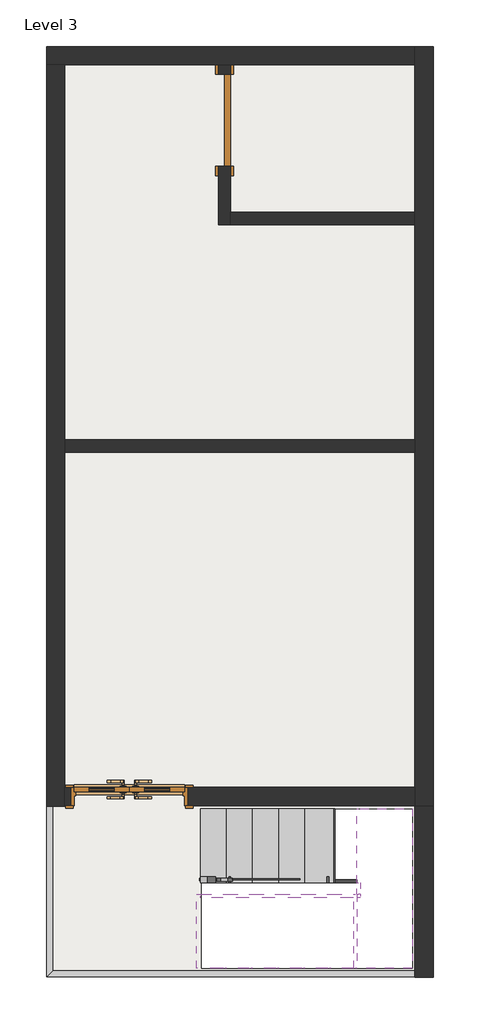
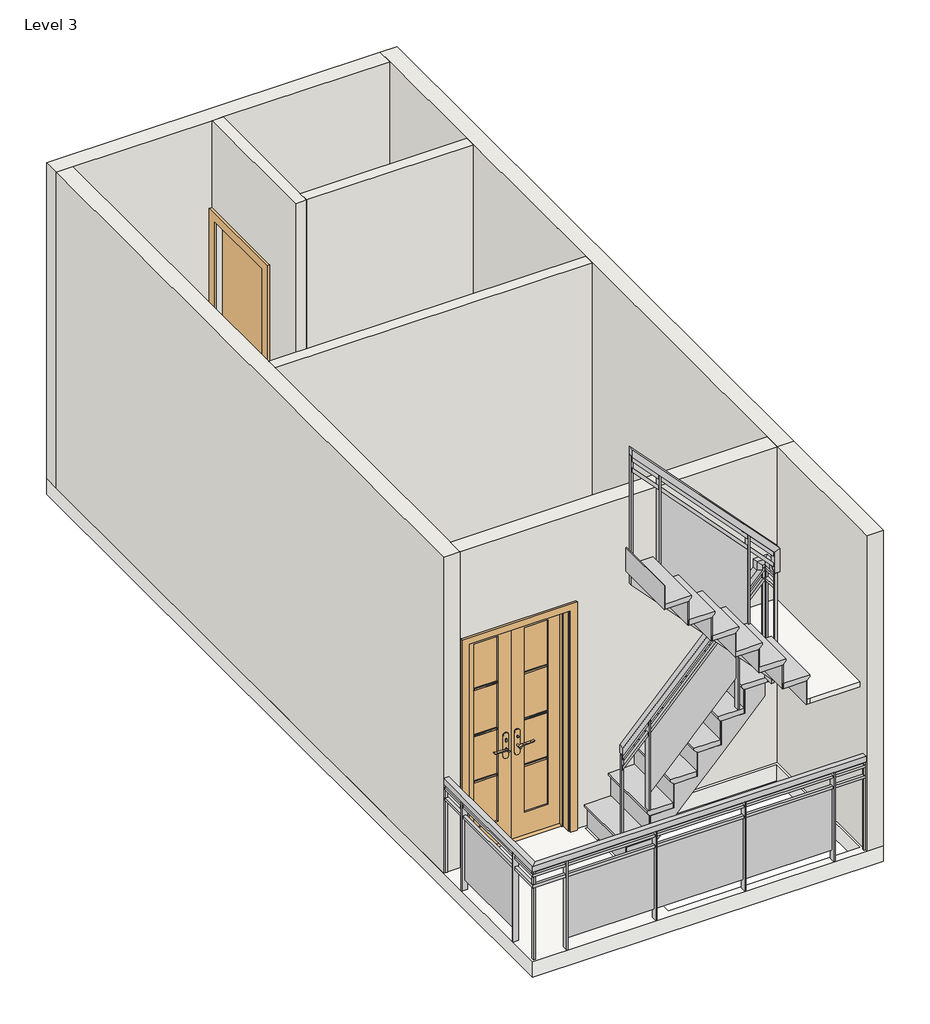
# One storey: 8 walls, 3 members, 2 doors, 2 railings, 2 slabs, 2 stair flights.
"""IFC4 building model written with IfcOpenShell, lengths in millimetres."""

from ifc_helpers import new_model, si_unit, frame, origin, place, context, project, spatial, polyline, outline, extrude, faceted_brep, transform, mapped, element, save
from components import door_665efd91, single_flush_2_5_aa9e95e7, non_monolithic_landing_1e13c623, stair_flight_b3ddc6eb, stair_flight_92f8819d

model = new_model("IFC4")

# Units and contexts
model_context = context("Model", 3, world=origin())
ifc_project = project(units=[si_unit("LENGTHUNIT", "METRE", prefix="MILLI")], contexts=[model_context])

# Site, building, storey
site = spatial("IfcSite", under=ifc_project)
building = spatial("IfcBuilding", under=site)
storey = spatial("IfcBuildingStorey", under=building, Name="Level 3", Elevation=6400.8)

# Doors
placement = place(None, origin())
door_shape = door_665efd91(model_context)
element("IfcDoor", 1, ObjectType="Door-Exterior-Double-Full Glass-Wood_Clad : 60\" x 84\"", at=placement, inside=storey, context=model_context, shape_type="MappedRepresentation", body=[
    mapped(door_shape, transform((-5617.280937, -3133.7029636, 6400.8), x_axis=(1.0, 0.0, 0.0), y_axis=(0.0, 1.0, 0.0), z_axis=(0.0, 0.0, 1.0))),
])
single_flush_2_5_shape = single_flush_2_5_aa9e95e7(model_context)
element("IfcDoor", 2, ObjectType="Single-Flush : 2.5'", at=placement, inside=storey, context=model_context, shape_type="MappedRepresentation", body=[
    mapped(single_flush_2_5_shape, transform((-4829.880937, 2455.4335625, 6400.8), x_axis=(0.0, 1.0, 0.0), y_axis=(-1.0, 0.0, 0.0), z_axis=(0.0, 0.0, 1.0))),
])

# Members
element("IfcMember", 3, ObjectType="Carriage - 2\" Width", at=placement, inside=storey, context=model_context, shape_type="Brep", body=[
    faceted_brep([(-4996.3909298, -3822.6779636, 6400.8), (-4861.0694778, -3822.6779636, 6400.8), (-4861.0694778, -3848.0779636, 6400.8), (-4996.3909298, -3848.0779636, 6400.8), (-3732.7409298, -3822.6779636, 7595.5008155), (-3732.7409298, -3848.0779636, 7595.5008155), (-3916.8909298, -3848.0779636, 7400.5184625), (-4132.7909298, -3848.0779636, 7171.9184625), (-4348.6909298, -3848.0779636, 6943.3184625), (-4564.5909298, -3848.0779636, 6714.7184625), (-4780.4909298, -3848.0779636, 6486.1184625), (-3732.7409298, -3822.6779636, 7721.6), (-4996.3909298, -3822.6779636, 6578.6), (-4780.4909298, -3822.6779636, 6578.6), (-4780.4909298, -3822.6779636, 6807.2), (-4564.5909298, -3822.6779636, 6807.2), (-4564.5909298, -3822.6779636, 7035.8), (-4348.6909298, -3822.6779636, 7035.8), (-4348.6909298, -3822.6779636, 7264.4), (-4132.7909298, -3822.6779636, 7264.4), (-4132.7909298, -3822.6779636, 7493.0), (-3916.8909298, -3822.6779636, 7493.0), (-3916.8909298, -3822.6779636, 7721.6), (-3916.8909298, -3848.0779636, 7721.6), (-3732.7409298, -3848.0779636, 7721.6), (-3916.8909298, -3848.0779636, 7493.0), (-4132.7909298, -3848.0779636, 7493.0), (-4132.7909298, -3848.0779636, 7264.4), (-4348.6909298, -3848.0779636, 7264.4), (-4348.6909298, -3848.0779636, 7035.8), (-4564.5909298, -3848.0779636, 7035.8), (-4564.5909298, -3848.0779636, 6807.2), (-4780.4909298, -3848.0779636, 6807.2), (-4780.4909298, -3848.0779636, 6578.6), (-4996.3909298, -3848.0779636, 6578.6)], [[[0, 1, 2, 3]], [[4, 5, 6, 7, 8, 9, 10, 2, 1]], [[11, 4, 1, 0, 12, 13, 14, 15, 16, 17, 18, 19, 20, 21, 22]], [[22, 23, 24, 11]], [[5, 24, 23, 25, 26, 27, 28, 29, 30, 31, 32, 33, 34, 3, 2, 10, 9, 8, 7, 6]], [[34, 12, 0, 3]], [[12, 34, 33, 13]], [[13, 33, 32, 14]], [[14, 32, 31, 15]], [[15, 31, 30, 16]], [[16, 30, 29, 17]], [[17, 29, 28, 18]], [[18, 28, 27, 19]], [[19, 27, 26, 20]], [[20, 26, 25, 21]], [[21, 25, 23, 22]], [[5, 4, 11, 24]]]),
])
element("IfcMember", 4, ObjectType="Carriage - 2\" Width", at=placement, inside=storey, context=model_context, shape_type="Brep", body=[
    faceted_brep([(-5028.1409298, -3945.3664375, 9195.7008155), (-5028.1409298, -3970.7664375, 9195.7008155), (-5028.1409298, -3970.7664375, 9321.8), (-5028.1409298, -3945.3664375, 9321.8), (-3707.3409298, -3970.7664375, 7797.2066978), (-3707.3409298, -3970.7664375, 7950.2), (-3764.4909298, -3970.7664375, 7950.2), (-3764.4909298, -3970.7664375, 8178.8), (-3980.3909298, -3970.7664375, 8178.8), (-3980.3909298, -3970.7664375, 8407.4), (-4196.2909298, -3970.7664375, 8407.4), (-4196.2909298, -3970.7664375, 8636.0), (-4412.1909298, -3970.7664375, 8636.0), (-4412.1909298, -3970.7664375, 8864.6), (-4628.0909298, -3970.7664375, 8864.6), (-4628.0909298, -3970.7664375, 9093.2), (-4843.9909298, -3970.7664375, 9093.2), (-4843.9909298, -3970.7664375, 9321.8), (-4843.9909298, -3945.3664375, 9000.7184625), (-4628.0909298, -3945.3664375, 8772.1184625), (-4412.1909298, -3945.3664375, 8543.5184625), (-4196.2909298, -3945.3664375, 8314.9184625), (-3980.3909298, -3945.3664375, 8086.3184625), (-3764.4909298, -3945.3664375, 7857.7184625), (-3732.7409298, -3945.3664375, 7824.1008155), (-3707.3409298, -3945.3664375, 7797.2066978), (-4843.9909298, -3945.3664375, 9321.8), (-4843.9909298, -3945.3664375, 9093.2), (-4628.0909298, -3945.3664375, 9093.2), (-4628.0909298, -3945.3664375, 8864.6), (-4412.1909298, -3945.3664375, 8864.6), (-4412.1909298, -3945.3664375, 8636.0), (-4196.2909298, -3945.3664375, 8636.0), (-4196.2909298, -3945.3664375, 8407.4), (-3980.3909298, -3945.3664375, 8407.4), (-3980.3909298, -3945.3664375, 8178.8), (-3764.4909298, -3945.3664375, 8178.8), (-3764.4909298, -3945.3664375, 7950.2), (-3732.7409298, -3945.3664375, 7950.2), (-3707.3409298, -3945.3664375, 7950.2)], [[[0, 1, 2, 3]], [[1, 4, 5, 6, 7, 8, 9, 10, 11, 12, 13, 14, 15, 16, 17, 2]], [[1, 0, 18, 19, 20, 21, 22, 23, 24, 25, 4]], [[0, 3, 26, 27, 28, 29, 30, 31, 32, 33, 34, 35, 36, 37, 38, 39, 25, 24, 23, 22, 21, 20, 19, 18]], [[7, 36, 35, 8]], [[36, 7, 6, 37]], [[9, 34, 33, 10]], [[8, 35, 34, 9]], [[11, 32, 31, 12]], [[10, 33, 32, 11]], [[13, 30, 29, 14]], [[12, 31, 30, 13]], [[15, 28, 27, 16]], [[14, 29, 28, 15]], [[17, 26, 3, 2]], [[16, 27, 26, 17]], [[4, 25, 39, 5]], [[37, 6, 5, 39, 38]]]),
])
element("IfcMember", 5, ObjectType="Carriage - 2\" Width", at=placement, inside=storey, context=model_context, shape_type="SweptSolid", body=[
    extrude(outline(polyline([(-3707.3409298, -3945.3664375), (-3732.7409298, -3945.3664375), (-3732.7409298, -3848.0779636), (-3707.3409298, -3848.0779636), (-3707.3409298, -3945.3664375)])), frame((0.0, 0.0, 7772.4), z_axis=(0.0, 0.0, 1.0), x_axis=(1.0, 0.0, 0.0)), (0.0, 0.0, 1.0), 177.8),
])

# Railings
element("IfcRailing", 6, ObjectType="Glass Panel - Bottom Fill", at=placement, inside=storey, context=model_context, shape_type="SolidModel", body=[
    faceted_brep([(-5028.1409298, -3797.2779636, 7543.8), (-5028.1409298, -3797.2779636, 7469.81477), (-5028.1409298, -3848.0779636, 7469.81477), (-5028.1409298, -3848.0779636, 7543.8), (-3808.9409298, -3797.2779636, 8834.7176471), (-3758.1409298, -3797.2779636, 8814.5206524), (-3758.1409298, -3848.0779636, 8814.5206524), (-3808.9409298, -3848.0779636, 8834.7176471), (-3681.9409298, -3945.3664375, 8915.4), (-3732.7409298, -3945.3664375, 8915.4), (-3732.7409298, -3996.1664375, 8864.6), (-3681.9409298, -3996.1664375, 8864.6), (-3681.9409298, -3924.2779636, 8864.6), (-3681.9409298, -3924.2779636, 8915.4), (-3732.7409298, -3924.2779636, 8864.6), (-3732.7409298, -3924.2779636, 8915.4), (-3808.9409298, -3797.2779636, 8915.4), (-3758.1409298, -3797.2779636, 8864.6), (-3758.1409298, -3848.0779636, 8864.6), (-3808.9409298, -3848.0779636, 8915.4), (-3681.9409298, -3797.2779636, 8915.4), (-3681.9409298, -3797.2779636, 8864.6), (-3732.7409298, -3848.0779636, 8864.6), (-3732.7409298, -3848.0779636, 8915.4)], [[[0, 1, 2, 3]], [[1, 0, 4, 5]], [[2, 1, 5, 6]], [[3, 2, 6, 7]], [[0, 3, 7, 4]], [[8, 9, 10, 11]], [[12, 13, 8, 11]], [[14, 12, 11, 10]], [[15, 14, 10, 9]], [[13, 15, 9, 8]], [[5, 4, 16, 17]], [[6, 5, 17, 18]], [[7, 6, 18, 19]], [[4, 7, 19, 16]], [[17, 16, 20, 21]], [[18, 17, 21, 22]], [[19, 18, 22, 23]], [[16, 19, 23, 20]], [[21, 20, 13, 12]], [[22, 21, 12, 14]], [[23, 22, 14, 15]], [[20, 23, 15, 13]]]),
    faceted_brep([(-3681.9409298, -3996.1664375, 9090.2117647), (-3732.7409298, -3996.1664375, 9070.01477), (-3732.7409298, -3945.3664375, 9070.01477), (-3681.9409298, -3945.3664375, 9090.2117647), (-5028.1409298, -3996.1664375, 10515.6), (-5028.1409298, -3945.3664375, 10515.6), (-5028.1409298, -3945.3664375, 10441.61477), (-5028.1409298, -3996.1664375, 10441.61477)], [[[0, 1, 2, 3]], [[4, 5, 6, 7]], [[1, 0, 4, 7]], [[2, 1, 7, 6]], [[3, 2, 6, 5]], [[0, 3, 5, 4]]]),
    faceted_brep([(-3681.9409298, -3945.3664375, 8915.4), (-3681.9409298, -3996.1664375, 8864.6), (-3732.7409298, -3996.1664375, 8864.6), (-3732.7409298, -3945.3664375, 8915.4), (-3681.9409298, -3945.3664375, 9090.2117647), (-3732.7409298, -3945.3664375, 9070.01477), (-3732.7409298, -3996.1664375, 9070.01477), (-3681.9409298, -3996.1664375, 9090.2117647)], [[[0, 1, 2, 3]], [[4, 5, 6, 7]], [[1, 0, 4, 7]], [[2, 1, 7, 6]], [[3, 2, 6, 5]], [[0, 3, 5, 4]]]),
    faceted_brep([(-5028.1409298, -3835.3779636, 7460.6963075), (-5028.1409298, -3809.9779636, 7460.6963075), (-5028.1409298, -3809.9779636, 7423.7036925), (-5028.1409298, -3835.3779636, 7423.7036925), (-3738.2152202, -3835.3779636, 8826.5), (-3738.2152202, -3809.9779636, 8826.5), (-3727.2666394, -3809.9779636, 8801.1), (-3727.2666394, -3835.3779636, 8801.1), (-3720.0409298, -3835.3779636, 8826.5), (-3694.6409298, -3809.9779636, 8826.5), (-3694.6409298, -3809.9779636, 8801.1), (-3720.0409298, -3835.3779636, 8801.1), (-3720.0409298, -3958.0664375, 8826.5), (-3720.0409298, -3958.0664375, 8801.1), (-3694.6409298, -3958.0664375, 8801.1), (-3694.6409298, -3958.0664375, 8826.5)], [[[0, 1, 2, 3]], [[1, 0, 4, 5]], [[2, 1, 5, 6]], [[3, 2, 6, 7]], [[0, 3, 7, 4]], [[5, 4, 8, 9]], [[6, 5, 9, 10]], [[7, 6, 10, 11]], [[4, 7, 11, 8]], [[12, 13, 14, 15]], [[9, 8, 12, 15]], [[10, 9, 15, 14]], [[11, 10, 14, 13]], [[8, 11, 13, 12]]]),
    faceted_brep([(-3694.6409298, -3958.0664375, 9020.555131), (-3694.6409298, -3983.4664375, 9020.555131), (-3694.6409298, -3983.4664375, 8983.562516), (-3694.6409298, -3958.0664375, 8983.562516), (-5028.1409298, -3958.0664375, 10432.4963075), (-5028.1409298, -3958.0664375, 10395.5036925), (-5028.1409298, -3983.4664375, 10395.5036925), (-5028.1409298, -3983.4664375, 10432.4963075)], [[[0, 1, 2, 3]], [[4, 5, 6, 7]], [[1, 0, 4, 7]], [[2, 1, 7, 6]], [[3, 2, 6, 5]], [[0, 3, 5, 4]]]),
    faceted_brep([(-5028.1409298, -3835.3779636, 7359.0963075), (-5028.1409298, -3809.9779636, 7359.0963075), (-5028.1409298, -3809.9779636, 7322.1036925), (-5028.1409298, -3835.3779636, 7322.1036925), (-3738.2152202, -3835.3779636, 8724.9), (-3738.2152202, -3809.9779636, 8724.9), (-3727.2666394, -3809.9779636, 8699.5), (-3727.2666394, -3835.3779636, 8699.5), (-3720.0409298, -3835.3779636, 8724.9), (-3694.6409298, -3809.9779636, 8724.9), (-3694.6409298, -3809.9779636, 8699.5), (-3720.0409298, -3835.3779636, 8699.5), (-3720.0409298, -3958.0664375, 8724.9), (-3720.0409298, -3958.0664375, 8699.5), (-3694.6409298, -3958.0664375, 8699.5), (-3694.6409298, -3958.0664375, 8724.9)], [[[0, 1, 2, 3]], [[1, 0, 4, 5]], [[2, 1, 5, 6]], [[3, 2, 6, 7]], [[0, 3, 7, 4]], [[5, 4, 8, 9]], [[6, 5, 9, 10]], [[7, 6, 10, 11]], [[4, 7, 11, 8]], [[12, 13, 14, 15]], [[9, 8, 12, 15]], [[10, 9, 15, 14]], [[11, 10, 14, 13]], [[8, 11, 13, 12]]]),
    faceted_brep([(-3694.6409298, -3958.0664375, 8918.955131), (-3694.6409298, -3983.4664375, 8918.955131), (-3694.6409298, -3983.4664375, 8881.962516), (-3694.6409298, -3958.0664375, 8881.962516), (-5028.1409298, -3958.0664375, 10330.8963075), (-5028.1409298, -3958.0664375, 10293.9036925), (-5028.1409298, -3983.4664375, 10293.9036925), (-5028.1409298, -3983.4664375, 10330.8963075)], [[[0, 1, 2, 3]], [[4, 5, 6, 7]], [[1, 0, 4, 7]], [[2, 1, 7, 6]], [[3, 2, 6, 5]], [[0, 3, 5, 4]]]),
    extrude(outline(polyline([(10165.9500641, -4767.7909298), (10179.397123, -4780.4909298), (9144.0, -4780.4909298), (9144.0, -4767.7909298), (10165.9500641, -4767.7909298)])), frame((0.0, -3996.1664375, 0.0), z_axis=(0.0, 1.0, 0.0), x_axis=(0.0, 0.0, 1.0)), (0.0, 0.0, 1.0), 50.8),
    extrude(outline(polyline([(8358.0941176, -3961.3409298), (9164.3507513, -3961.3409298), (10024.962516, -4774.1409298), (9218.7058824, -4774.1409298), (8358.0941176, -3961.3409298)])), frame((0.0, -3977.3015945, 0.0), z_axis=(0.0, 1.0, 0.0), x_axis=(0.0, 0.0, 1.0)), (0.0, 0.0, 1.0), 6.35),
    extrude(outline(polyline([(9305.3382994, -3954.9909298), (9318.7853582, -3967.6909298), (8458.2, -3967.6909298), (8458.2, -3954.9909298), (9305.3382994, -3954.9909298)])), frame((0.0, -3996.1664375, 0.0), z_axis=(0.0, 1.0, 0.0), x_axis=(0.0, 0.0, 1.0)), (0.0, 0.0, 1.0), 50.8),
    extrude(outline(polyline([(8592.6441818, -3967.6909298), (8579.197123, -3980.3909298), (7543.8, -3980.3909298), (7543.8, -3967.6909298), (8592.6441818, -3967.6909298)])), frame((0.0, -3848.0779636, 0.0), z_axis=(0.0, 1.0, 0.0), x_axis=(0.0, 0.0, 1.0)), (0.0, 0.0, 1.0), 50.8),
    extrude(outline(polyline([(6986.4941176, -4786.8409298), (7847.1058824, -3974.0409298), (8438.2095749, -3974.0409298), (7577.5978102, -4786.8409298), (6986.4941176, -4786.8409298)])), frame((0.0, -3822.4928066, 0.0), z_axis=(0.0, 1.0, 0.0), x_axis=(0.0, 0.0, 1.0)), (0.0, 0.0, 1.0), 6.35),
    extrude(outline(polyline([(7732.0324171, -4780.4909298), (7718.5853582, -4793.1909298), (6858.0, -4793.1909298), (6858.0, -4780.4909298), (7732.0324171, -4780.4909298)])), frame((0.0, -3848.0779636, 0.0), z_axis=(0.0, 1.0, 0.0), x_axis=(0.0, 0.0, 1.0)), (0.0, 0.0, 1.0), 50.8),
    extrude(outline(polyline([(-3697.8159298, -3961.2414375), (-3697.8159298, -3980.2914375), (-3716.8659298, -3980.2914375), (-3716.8659298, -3961.2414375), (-3697.8159298, -3961.2414375)])), frame((0.0, 0.0, 8001.0), z_axis=(0.0, 0.0, 1.0), x_axis=(1.0, 0.0, 0.0)), (0.0, 0.0, 1.0), 863.6),
    extrude(outline(polyline([(-3716.8659298, -3832.2029636), (-3716.8659298, -3813.1529636), (-3697.8159298, -3813.1529636), (-3697.8159298, -3832.2029636), (-3716.8659298, -3832.2029636)])), frame((0.0, 0.0, 8001.0), z_axis=(0.0, 0.0, 1.0), x_axis=(1.0, 0.0, 0.0)), (0.0, 0.0, 1.0), 863.6),
    extrude(outline(polyline([(-3742.2659298, -3832.2029636), (-3742.2659298, -3813.1529636), (-3723.2159298, -3813.1529636), (-3723.2159298, -3832.2029636), (-3742.2659298, -3832.2029636)])), frame((0.0, 0.0, 8001.0), z_axis=(0.0, 0.0, 1.0), x_axis=(1.0, 0.0, 0.0)), (0.0, 0.0, 1.0), 863.6),
    extrude(outline(polyline([(10428.1677112, -5015.4409298), (10448.3382994, -5034.4909298), (9372.6, -5034.4909298), (9372.6, -5015.4409298), (10428.1677112, -5015.4409298)])), frame((0.0, -3980.2914375, 0.0), z_axis=(0.0, 1.0, 0.0), x_axis=(0.0, 0.0, 1.0)), (0.0, 0.0, 1.0), 19.05),
    extrude(outline(polyline([(7483.2618288, -5015.4409298), (7463.0912406, -5034.4909298), (6629.4, -5034.4909298), (6629.4, -5015.4409298), (7483.2618288, -5015.4409298)])), frame((0.0, -3832.2029636, 0.0), z_axis=(0.0, 1.0, 0.0), x_axis=(0.0, 0.0, 1.0)), (0.0, 0.0, 1.0), 19.05),
])
element("IfcRailing", 7, ObjectType="Glass Panel - Bottom Fill", at=placement, inside=storey, context=model_context, shape_type="SolidModel", body=[
    faceted_brep([(-6252.280937, -3208.7664375, 7315.2), (-6252.280937, -3208.7664375, 7264.4), (-6303.080937, -3208.7664375, 7264.4), (-6303.080937, -3208.7664375, 7315.2), (-6252.280937, -4574.0164375, 7315.2), (-6252.280937, -4574.0164375, 7264.4), (-6303.080937, -4624.8164375, 7264.4), (-6303.080937, -4624.8164375, 7315.2), (-3255.080937, -4574.0164375, 7315.2), (-3255.080937, -4624.8164375, 7315.2), (-3255.080937, -4624.8164375, 7264.4), (-3255.080937, -4574.0164375, 7264.4)], [[[0, 1, 2, 3]], [[1, 0, 4, 5]], [[2, 1, 5, 6]], [[3, 2, 6, 7]], [[0, 3, 7, 4]], [[8, 9, 10, 11]], [[5, 4, 8, 11]], [[6, 5, 11, 10]], [[7, 6, 10, 9]], [[4, 7, 9, 8]]]),
    faceted_brep([(-6290.380937, -3208.7664375, 7226.3), (-6264.980937, -3208.7664375, 7226.3), (-6264.980937, -3208.7664375, 7200.9), (-6290.380937, -3208.7664375, 7200.9), (-6290.380937, -4612.1164375, 7226.3), (-6264.980937, -4586.7164375, 7226.3), (-6264.980937, -4586.7164375, 7200.9), (-6290.380937, -4612.1164375, 7200.9), (-3255.080937, -4612.1164375, 7226.3), (-3255.080937, -4612.1164375, 7200.9), (-3255.080937, -4586.7164375, 7200.9), (-3255.080937, -4586.7164375, 7226.3)], [[[0, 1, 2, 3]], [[1, 0, 4, 5]], [[2, 1, 5, 6]], [[3, 2, 6, 7]], [[0, 3, 7, 4]], [[8, 9, 10, 11]], [[5, 4, 8, 11]], [[6, 5, 11, 10]], [[7, 6, 10, 9]], [[4, 7, 9, 8]]]),
    faceted_brep([(-6290.380937, -3208.7664375, 7124.7), (-6264.980937, -3208.7664375, 7124.7), (-6264.980937, -3208.7664375, 7099.3), (-6290.380937, -3208.7664375, 7099.3), (-6290.380937, -4612.1164375, 7124.7), (-6264.980937, -4586.7164375, 7124.7), (-6264.980937, -4586.7164375, 7099.3), (-6290.380937, -4612.1164375, 7099.3), (-3255.080937, -4612.1164375, 7124.7), (-3255.080937, -4612.1164375, 7099.3), (-3255.080937, -4586.7164375, 7099.3), (-3255.080937, -4586.7164375, 7124.7)], [[[0, 1, 2, 3]], [[1, 0, 4, 5]], [[2, 1, 5, 6]], [[3, 2, 6, 7]], [[0, 3, 7, 4]], [[8, 9, 10, 11]], [[5, 4, 8, 11]], [[6, 5, 11, 10]], [[7, 6, 10, 9]], [[4, 7, 9, 8]]]),
    extrude(outline(polyline([(-3553.530937, -4624.8164375), (-3553.530937, -4574.0164375), (-3540.830937, -4574.0164375), (-3540.830937, -4624.8164375), (-3553.530937, -4624.8164375)])), frame((0.0, 0.0, 6400.8), z_axis=(0.0, 0.0, 1.0), x_axis=(1.0, 0.0, 0.0)), (0.0, 0.0, 1.0), 863.6),
    extrude(outline(polyline([(-4359.980937, -4592.8812805), (-3547.180937, -4592.8812805), (-3547.180937, -4599.2312805), (-4359.980937, -4599.2312805), (-4359.980937, -4592.8812805)])), frame((0.0, 0.0, 6502.4), z_axis=(0.0, 0.0, 1.0), x_axis=(1.0, 0.0, 0.0)), (0.0, 0.0, 1.0), 596.9),
    extrude(outline(polyline([(-4366.330937, -4624.8164375), (-4366.330937, -4574.0164375), (-4353.630937, -4574.0164375), (-4353.630937, -4624.8164375), (-4366.330937, -4624.8164375)])), frame((0.0, 0.0, 6400.8), z_axis=(0.0, 0.0, 1.0), x_axis=(1.0, 0.0, 0.0)), (0.0, 0.0, 1.0), 863.6),
    extrude(outline(polyline([(-5172.780937, -4592.8812805), (-4359.980937, -4592.8812805), (-4359.980937, -4599.2312805), (-5172.780937, -4599.2312805), (-5172.780937, -4592.8812805)])), frame((0.0, 0.0, 6502.4), z_axis=(0.0, 0.0, 1.0), x_axis=(1.0, 0.0, 0.0)), (0.0, 0.0, 1.0), 596.9),
    extrude(outline(polyline([(-5179.130937, -4624.8164375), (-5179.130937, -4574.0164375), (-5166.430937, -4574.0164375), (-5166.430937, -4624.8164375), (-5179.130937, -4624.8164375)])), frame((0.0, 0.0, 6400.8), z_axis=(0.0, 0.0, 1.0), x_axis=(1.0, 0.0, 0.0)), (0.0, 0.0, 1.0), 863.6),
    extrude(outline(polyline([(-5985.580937, -4592.8812805), (-5172.780937, -4592.8812805), (-5172.780937, -4599.2312805), (-5985.580937, -4599.2312805), (-5985.580937, -4592.8812805)])), frame((0.0, 0.0, 6502.4), z_axis=(0.0, 0.0, 1.0), x_axis=(1.0, 0.0, 0.0)), (0.0, 0.0, 1.0), 596.9),
    extrude(outline(polyline([(-5991.930937, -4624.8164375), (-5991.930937, -4574.0164375), (-5979.230937, -4574.0164375), (-5979.230937, -4624.8164375), (-5991.930937, -4624.8164375)])), frame((0.0, 0.0, 6400.8), z_axis=(0.0, 0.0, 1.0), x_axis=(1.0, 0.0, 0.0)), (0.0, 0.0, 1.0), 863.6),
    extrude(outline(polyline([(-6303.080937, -4304.1414375), (-6252.280937, -4304.1414375), (-6252.280937, -4316.8414375), (-6303.080937, -4316.8414375), (-6303.080937, -4304.1414375)])), frame((0.0, 0.0, 6400.8), z_axis=(0.0, 0.0, 1.0), x_axis=(1.0, 0.0, 0.0)), (0.0, 0.0, 1.0), 863.6),
    extrude(outline(polyline([(-6271.14578, -3497.6914375), (-6271.14578, -4310.4914375), (-6277.49578, -4310.4914375), (-6277.49578, -3497.6914375), (-6271.14578, -3497.6914375)])), frame((0.0, 0.0, 6502.4), z_axis=(0.0, 0.0, 1.0), x_axis=(1.0, 0.0, 0.0)), (0.0, 0.0, 1.0), 596.9),
    extrude(outline(polyline([(-6303.080937, -3491.3414375), (-6252.280937, -3491.3414375), (-6252.280937, -3504.0414375), (-6303.080937, -3504.0414375), (-6303.080937, -3491.3414375)])), frame((0.0, 0.0, 6400.8), z_axis=(0.0, 0.0, 1.0), x_axis=(1.0, 0.0, 0.0)), (0.0, 0.0, 1.0), 863.6),
    extrude(outline(polyline([(-6287.205937, -4589.8914375), (-6268.155937, -4589.8914375), (-6268.155937, -4608.9414375), (-6287.205937, -4608.9414375), (-6287.205937, -4589.8914375)])), frame((0.0, 0.0, 6400.8), z_axis=(0.0, 0.0, 1.0), x_axis=(1.0, 0.0, 0.0)), (0.0, 0.0, 1.0), 863.6),
    extrude(outline(polyline([(-3267.780937, -4608.9414375), (-3267.780937, -4589.8914375), (-3248.730937, -4589.8914375), (-3248.730937, -4608.9414375), (-3267.780937, -4608.9414375)])), frame((0.0, 0.0, 6400.8), z_axis=(0.0, 0.0, 1.0), x_axis=(1.0, 0.0, 0.0)), (0.0, 0.0, 1.0), 863.6),
    extrude(outline(polyline([(-6287.205937, -3202.4164375), (-6268.155937, -3202.4164375), (-6268.155937, -3221.4664375), (-6287.205937, -3221.4664375), (-6287.205937, -3202.4164375)])), frame((0.0, 0.0, 6400.8), z_axis=(0.0, 0.0, 1.0), x_axis=(1.0, 0.0, 0.0)), (0.0, 0.0, 1.0), 863.6),
])

# Slabs
element("IfcSlab", 8, ObjectType="6\"", at=placement, inside=storey, context=model_context, shape_type="SweptSolid", body=[
    extrude(outline(polyline([(-3102.680937, 3065.0335625), (-3102.680937, -4624.8164375), (-6303.080937, -4624.8164375), (-6303.080937, 3065.0335625), (-3102.680937, 3065.0335625)]), holes=[polyline([(-5021.7909298, -3238.4779636), (-5021.7909298, -4554.9664375), (-3275.5409298, -4554.9664375), (-3275.5409298, -3238.4779636), (-5021.7909298, -3238.4779636)])]), frame((0.0, 0.0, 6248.4), z_axis=(0.0, 0.0, 1.0), x_axis=(1.0, 0.0, 0.0)), (0.0, 0.0, 1.0), 152.4),
])
non_monolithic_landing_shape = non_monolithic_landing_1e13c623(model_context)
element("IfcSlab", 9, ObjectType="Non-Monolithic Landing", at=placement, inside=storey, context=model_context, shape_type="MappedRepresentation", body=[
    mapped(non_monolithic_landing_shape, transform((0.0, 0.0, 0.0), x_axis=(1.0, 0.0, 0.0), y_axis=(0.0, 1.0, 0.0), z_axis=(0.0, 0.0, 1.0))),
])

# Stair flights
stair_flight_shape = stair_flight_b3ddc6eb(model_context)
element("IfcStairFlight", 10, ObjectType="2\" Tread 1\" Nosing 1/4\" Riser", at=placement, inside=storey, context=model_context, shape_type="MappedRepresentation", body=[
    mapped(stair_flight_shape, transform((0.0, 0.0, 0.0), x_axis=(1.0, 0.0, 0.0), y_axis=(0.0, 1.0, 0.0), z_axis=(0.0, 0.0, 1.0))),
])
stair_flight_2_shape = stair_flight_92f8819d(model_context)
element("IfcStairFlight", 11, ObjectType="2\" Tread 1\" Nosing 1/4\" Riser", at=placement, inside=storey, context=model_context, shape_type="MappedRepresentation", body=[
    mapped(stair_flight_2_shape, transform((0.0, 0.0, 0.0), x_axis=(1.0, 0.0, 0.0), y_axis=(0.0, 1.0, 0.0), z_axis=(0.0, 0.0, 1.0))),
])

# Walls
element("IfcWall", 12, ObjectType="4\"", at=placement, inside=storey, context=model_context, shape_type="Brep", body=[
    faceted_brep([(-4880.680937, 2912.6335625, 6400.8), (-4880.680937, 2836.4335625, 6400.8), (-4880.680937, 2836.4335625, 8534.4), (-4880.680937, 2074.4335625, 8534.4), (-4880.680937, 2074.4335625, 6400.8), (-4880.680937, 1591.8335625, 6400.8), (-4880.680937, 1591.8335625, 9448.8), (-4880.680937, 2912.6335625, 9448.8), (-4779.080937, 2836.4335625, 8534.4), (-4779.080937, 2836.4335625, 6400.8), (-4779.080937, 2912.6335625, 6400.8), (-4779.080937, 2912.6335625, 9448.8), (-4779.080937, 1693.4335625, 9448.8), (-4779.080937, 1591.8335625, 9448.8), (-4779.080937, 1591.8335625, 6400.8), (-4779.080937, 1693.4335625, 6400.8), (-4779.080937, 2074.4335625, 6400.8), (-4779.080937, 2074.4335625, 8534.4)], [[[0, 1, 2, 3, 4, 5, 6, 7]], [[8, 9, 10, 11, 12, 13, 14, 15, 16, 17]], [[10, 9, 1, 0]], [[16, 15, 14, 5, 4]], [[7, 6, 13, 12, 11]], [[0, 7, 11, 10]], [[6, 5, 14, 13]], [[2, 1, 9, 8]], [[3, 2, 8, 17]], [[4, 3, 17, 16]]]),
])
element("IfcWall", 13, ObjectType="4\"", at=placement, inside=storey, context=model_context, shape_type="SweptSolid", body=[
    extrude(outline(polyline([(-3255.080937, 1591.8335625), (-4779.080937, 1591.8335625), (-4779.080937, 1693.4335625), (-3255.080937, 1693.4335625), (-3255.080937, 1591.8335625)])), frame((0.0, 0.0, 6400.8), z_axis=(0.0, 0.0, 1.0), x_axis=(1.0, 0.0, 0.0)), (0.0, 0.0, 1.0), 3048.0),
])
element("IfcWall", 14, ObjectType="4\"", at=placement, inside=storey, context=model_context, shape_type="SweptSolid", body=[
    extrude(outline(polyline([(-6150.680937, -186.1664375), (-3255.080937, -186.1664375), (-3255.080937, -287.7664375), (-6150.680937, -287.7664375), (-6150.680937, -186.1664375)])), frame((0.0, 0.0, 6400.8), z_axis=(0.0, 0.0, 1.0), x_axis=(1.0, 0.0, 0.0)), (0.0, 0.0, 1.0), 3048.0),
])
element("IfcWall", 15, ObjectType="6\"", at=placement, inside=storey, context=model_context, shape_type="Brep", body=[
    faceted_brep([(-6303.080937, 2912.6335625, 6400.8), (-6150.680937, 2912.6335625, 6400.8), (-4880.680937, 2912.6335625, 6400.8), (-4779.080937, 2912.6335625, 6400.8), (-3255.080937, 2912.6335625, 6400.8), (-3255.080937, 2912.6335625, 9448.8), (-4779.080937, 2912.6335625, 9448.8), (-4880.680937, 2912.6335625, 9448.8), (-6150.680937, 2912.6335625, 9448.8), (-6303.080937, 2912.6335625, 9448.8), (-6303.080937, 3065.0335625, 6400.8), (-6303.080937, 3065.0335625, 9448.8), (-3255.080937, 3065.0335625, 9448.8), (-3255.080937, 3065.0335625, 6400.8)], [[[0, 1, 2, 3, 4, 5, 6, 7, 8, 9]], [[10, 11, 12, 13]], [[4, 3, 2, 1, 0, 10, 13]], [[9, 8, 7, 6, 5, 12, 11]], [[0, 9, 11, 10]], [[5, 4, 13, 12]]]),
])
element("IfcWall", 16, ObjectType="6\"", at=placement, inside=storey, context=model_context, shape_type="Brep", body=[
    faceted_brep([(-3255.080937, 3065.0335625, 6400.8), (-3255.080937, 2912.6335625, 6400.8), (-3255.080937, 1693.4335625, 6400.8), (-3255.080937, 1591.8335625, 6400.8), (-3255.080937, -186.1664375, 6400.8), (-3255.080937, -287.7664375, 6400.8), (-3255.080937, -3060.6779636, 6400.8), (-3255.080937, -3213.0779636, 6400.8), (-3255.080937, -3215.1164375, 6400.8), (-3255.080937, -3215.1164375, 9448.8), (-3255.080937, -3213.0779636, 9448.8), (-3255.080937, -3060.6779636, 9448.8), (-3255.080937, -287.7664375, 9448.8), (-3255.080937, -186.1664375, 9448.8), (-3255.080937, 1591.8335625, 9448.8), (-3255.080937, 1693.4335625, 9448.8), (-3255.080937, 2912.6335625, 9448.8), (-3255.080937, 3065.0335625, 9448.8), (-3102.680937, 3065.0335625, 6400.8), (-3102.680937, 3065.0335625, 9448.8), (-3102.680937, -3215.1164375, 9448.8), (-3102.680937, -3215.1164375, 6400.8)], [[[0, 1, 2, 3, 4, 5, 6, 7, 8, 9, 10, 11, 12, 13, 14, 15, 16, 17]], [[18, 19, 20, 21]], [[8, 7, 6, 5, 4, 3, 2, 1, 0, 18, 21]], [[9, 8, 21, 20]], [[17, 16, 15, 14, 13, 12, 11, 10, 9, 20, 19]], [[0, 17, 19, 18]]]),
])
element("IfcWall", 17, ObjectType="6\"", at=placement, inside=storey, context=model_context, shape_type="SweptSolid", body=[
    extrude(outline(polyline([(9448.8, -3255.080937), (9448.8, -6150.680937), (6400.8, -6150.680937), (6400.8, -6099.880937), (8559.8, -6099.880937), (8559.8, -5134.680937), (6400.8, -5134.680937), (6400.8, -3255.080937), (9448.8, -3255.080937)])), frame((0.0, -3213.0779636, 0.0), z_axis=(0.0, 1.0, 0.0), x_axis=(0.0, 0.0, 1.0)), (0.0, 0.0, 1.0), 152.4),
])
element("IfcWall", 18, ObjectType="6\"", at=placement, inside=storey, context=model_context, shape_type="Brep", body=[
    faceted_brep([(-6150.680937, -3215.1164375, 6400.8), (-6150.680937, -3213.0779636, 6400.8), (-6150.680937, -3060.6779636, 6400.8), (-6150.680937, -287.7664375, 6400.8), (-6150.680937, -186.1664375, 6400.8), (-6150.680937, 2912.6335625, 6400.8), (-6150.680937, 2912.6335625, 9448.8), (-6150.680937, -186.1664375, 9448.8), (-6150.680937, -287.7664375, 9448.8), (-6150.680937, -3060.6779636, 9448.8), (-6150.680937, -3213.0779636, 9448.8), (-6150.680937, -3215.1164375, 9448.8), (-6303.080937, -3215.1164375, 6400.8), (-6303.080937, -3215.1164375, 9448.8), (-6303.080937, 2912.6335625, 9448.8), (-6303.080937, 2912.6335625, 6400.8)], [[[0, 1, 2, 3, 4, 5, 6, 7, 8, 9, 10, 11]], [[12, 13, 14, 15]], [[5, 4, 3, 2, 1, 0, 12, 15]], [[11, 10, 9, 8, 7, 6, 14, 13]], [[0, 11, 13, 12]], [[6, 5, 15, 14]]]),
])
element("IfcWall", 19, ObjectType="6\"", at=placement, inside=storey, context=model_context, shape_type="SweptSolid", body=[
    extrude(outline(polyline([(-3255.080937, -4631.1664375), (-3255.080937, -3215.1164375), (-3102.680937, -3215.1164375), (-3102.680937, -4631.1664375), (-3255.080937, -4631.1664375)])), frame((0.0, 0.0, 6400.8), z_axis=(0.0, 0.0, 1.0), x_axis=(1.0, 0.0, 0.0)), (0.0, 0.0, 1.0), 3048.0),
])

save(model, "model.ifc")

# Revit data of these elements
# Type "Door-Exterior-Double-Full Glass-Wood_Clad : 60\" x 84\""
#   Type Mark = "8"
#   Assembly Code = "B2030100"
#   Analytic Construction = "French door, wood frame with double glass"
#   Top Rail = 0' - 4 11/16"
#   Threshold Offset [instance default] = 0' - 0 1/2"
#   Thickness = 0' - 1 3/8"
#   Thermal Resistance (R) = 1.9158 (h·ft²·°F)/BTU
#   Swing Angle [instance default] = 90.00°
#   Stiles = 0' - 4 3/4"
#   Rough Width = 3' - 2"
#   Rough Height = 7' - 1"
#   Panel Width = 1' - 6"
#   Door Offset [instance default] = 0' - 0"
#   Height = 7' - 0"
#   Width = 3' - 0"
#   Heat Transfer Coefficient (U) = 0.5220 BTU/(h·ft²·°F)
#   Bottom Rail = 0' - 9 1/8"
#   Exterior Trim [instance default] = yes
#   Threshold [instance default] = yes
#   Show Grill [instance default] = yes
#   Function = 1
#   Trim Material = Cherry
#   Threshold Material = Cherry
#   Panel Material = Cherry
#   Glazing = Glass
#   Frame Material = Cherry
#   Door Handle Material = Aluminum
#   Visual Light Transmittance = 0
#   Solar Heat Gain Coefficient = 0
#   Wall Closure = (empty or 0)
#   Construction Type = (empty or 0)
# Type "Single-Flush : 2.5'"
#   Type Mark = "9"
#   Construction Type Id = "MDOOR"
#   Assembly Code = "C1020"
#   Analytic Construction = "Metal"
#   Thickness = 0' - 2"
#   Heat Transfer Coefficient (U) = 0.651978 BTU/(h·ft²·°F)
#   Height = 7' - 0"
#   Trim Projection Ext = 0' - 1"
#   Trim Projection Int = 0' - 1"
#   Trim Width = 0' - 3"
#   Width = 2' - 6"
#   Define Thermal Properties by = 1
#   Door Material = Door - Panel
#   Frame Material = Door - Frame
#   Visual Light Transmittance = 0
#   Solar Heat Gain Coefficient = 0
#   Function = (empty or 0)
#   Wall Closure = (empty or 0)
# Type "Glass Panel - Bottom Fill"
#   Assembly Code = "C2010400"
#   built-in parameter 1008612 = 0.0416667 (stored number, unit not read)
#   built-in parameter 1008611 = 0.0416667 (stored number, unit not read)
#   built-in parameter 1008609 = 0.333333 (stored number, unit not read)
#   built-in parameter 1008604 = 0.166667 (stored number, unit not read)
#   built-in parameter 1008603 = 0.166667 (stored number, unit not read)
#   Railing Height = 3' - 0"
#   built-in parameter 1008630 = 2
#   built-in parameter 1008610 = 2
#   built-in parameter 1008618 = Baluster - Square : 3/4"
# Type "6\""
#   Assembly Code = "B1010"
#   Function = 0
#   Layers, outside or top first: 0' - 6" no material (function 1)
# Type "4\""
#   Assembly Code = "B2010"
#   Layers, outside or top first: 0' - 4" no material (function 1)
# Type "6\""
#   Assembly Code = "B2010"
#   Layers, outside or top first: 0' - 6" no material (function 1)
# Element 1 (IfcDoor, "Door-Exterior-Double-Full Glass-Wood_Clad : 60\" x 84\"")
#   Threshold Offset = 0' - 0 1/2"
#   Swing Angle = 90.00°
#   Door Offset = 0' - 0"
#   Threshold = yes
#   Show Grill = yes
#   Exterior Trim = yes
#   Phase Created = New Construction
#   Materials on its faces: "Cherry", "Aluminum", "Glass"
# Element 2 (IfcDoor, "Single-Flush : 2.5'")
#   Phase Created = New Construction
#   Materials on its faces: "Door - Frame", "Door - Panel"
# Elements 3, 4, 5 (IfcMember, "Carriage - 2\" Width")
#   Phase Created = New Construction
# Elements 6, 7 (IfcRailing, "Glass Panel - Bottom Fill")
#   Phase Created = New Construction
#   Materials on its faces: "Glass"
# Element 8 (IfcSlab, "6\"")
#   Height Offset From Level = 0' - 0"
#   Phase Created = New Construction
#   Materials on its faces: "Default Floor"
# Element 9 (IfcSlab, "Non-Monolithic Landing")
#   Phase Created = New Construction
# Elements 10, 11 (IfcStairFlight, "2\" Tread 1\" Nosing 1/4\" Riser")
#   Phase Created = New Construction
# Elements 12, 13, 14 (IfcWall, "4\"")
#   Top Offset = 0' - 0"
#   Base Offset = 0' - 0"
#   Unconnected Height = 10' - 0"
#   wall height = 10' - 0"
#   Phase Created = New Construction
#   Base Constraint = Level 3
#   Materials on its faces: "Default Wall"
# Elements 15, 16, 17, 18, 19 (IfcWall, "6\"")
#   Top Offset = 0' - 0"
#   Base Offset = 0' - 0"
#   Unconnected Height = 10' - 0"
#   wall height = 10' - 0"
#   Phase Created = New Construction
#   Base Constraint = Level 3
#   Materials on its faces: "Default Wall"
# Materials
#   "Cherry": class "Wood", colour RGB 226 177 128, transparency 0, Description = "Prunus Serotina", Cost = 0
#   "Glass": class "Glass", colour RGB 0 128 192, transparency 0.75, Description = "Soda Lime Glass", Cost = 0
#   "Aluminum": class "Metal", colour RGB 247 247 247, transparency 0, Description = "Aluminum 6061", Cost = 0
#   "Door - Panel": class "Wood", colour RGB 210 159 95, transparency 0
#   "Door - Frame": colour RGB 118 70 51, transparency 0
#   "Default Floor": colour RGB 128 128 128, transparency 0
#   "Default Wall": colour RGB 128 128 128, transparency 0
